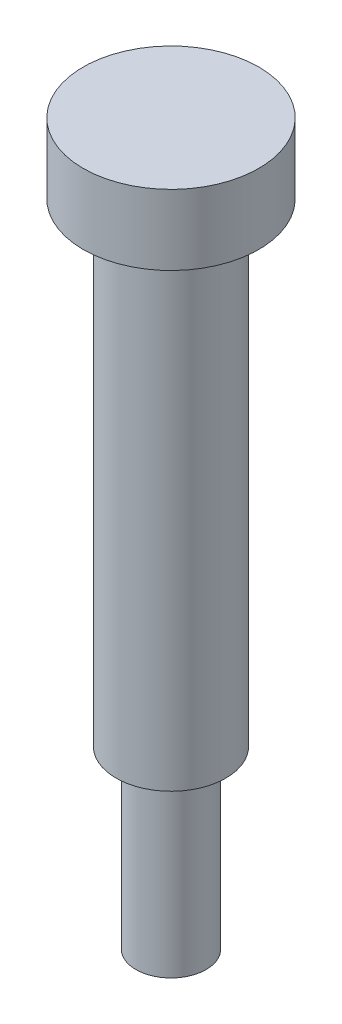
ISO-10303-21;
HEADER;
FILE_DESCRIPTION(('STEP AP214'),'2;1');
FILE_NAME('part.step','',(''),(''),'','','');
FILE_SCHEMA(('AUTOMOTIVE_DESIGN { 1 0 10303 214 1 1 1 1 }'));
ENDSEC;
DATA;
#1=APPLICATION_CONTEXT('core data for automotive mechanical design processes');
#2=APPLICATION_PROTOCOL_DEFINITION('international standard','automotive_design',2000,#1);
#3=PRODUCT_CONTEXT('',#1,'mechanical');
#4=PRODUCT('Part','Part','',(#3));
#5=PRODUCT_RELATED_PRODUCT_CATEGORY('part','',(#4));
#6=PRODUCT_DEFINITION_FORMATION('','',#4);
#7=PRODUCT_DEFINITION_CONTEXT('part definition',#1,'design');
#8=PRODUCT_DEFINITION('design','',#6,#7);
#9=PRODUCT_DEFINITION_SHAPE('','',#8);
#10=(LENGTH_UNIT() NAMED_UNIT(*) SI_UNIT(.MILLI.,.METRE.));
#11=(NAMED_UNIT(*) PLANE_ANGLE_UNIT() SI_UNIT($,.RADIAN.));
#12=(NAMED_UNIT(*) SI_UNIT($,.STERADIAN.) SOLID_ANGLE_UNIT());
#13=UNCERTAINTY_MEASURE_WITH_UNIT(LENGTH_MEASURE(1.E-05),#10,'distance_accuracy_value','');
#14=(GEOMETRIC_REPRESENTATION_CONTEXT(3) GLOBAL_UNCERTAINTY_ASSIGNED_CONTEXT((#13)) GLOBAL_UNIT_ASSIGNED_CONTEXT((#10,
#11,#12)) REPRESENTATION_CONTEXT('',''));
#15=CARTESIAN_POINT('',(0.,0.,0.));
#16=DIRECTION('',(0.,0.,1.));
#17=DIRECTION('',(1.,0.,0.));
#18=AXIS2_PLACEMENT_3D('',#15,#16,#17);
#19=CARTESIAN_POINT('',(0.,41.,0.));
#20=DIRECTION('',(0.,-1.,0.));
#21=DIRECTION('',(0.,0.,-1.));
#22=AXIS2_PLACEMENT_3D('',#19,#20,#21);
#23=PLANE('',#22);
#24=CARTESIAN_POINT('',(0.,41.,0.));
#25=DIRECTION('',(0.,-1.,0.));
#26=DIRECTION('',(0.,0.,-1.));
#27=AXIS2_PLACEMENT_3D('',#24,#25,#26);
#28=CIRCLE('',#27,5.);
#29=CARTESIAN_POINT('',(0.,41.,-5.));
#30=VERTEX_POINT('',#29);
#31=EDGE_CURVE('E10',#30,#30,#28,.T.);
#32=ORIENTED_EDGE('',*,*,#31,.F.);
#33=EDGE_LOOP('',(#32));
#34=FACE_BOUND('',#33,.T.);
#35=ADVANCED_FACE('F41',(#34),#23,.F.);
#36=CARTESIAN_POINT('',(0.,0.,0.));
#37=DIRECTION('',(0.,-1.,0.));
#38=DIRECTION('',(0.,0.,-1.));
#39=AXIS2_PLACEMENT_3D('',#36,#37,#38);
#40=CYLINDRICAL_SURFACE('',#39,5.);
#41=CARTESIAN_POINT('',(0.,37.,0.));
#42=DIRECTION('',(0.,-1.,0.));
#43=DIRECTION('',(0.,0.,-1.));
#44=AXIS2_PLACEMENT_3D('',#41,#42,#43);
#45=CIRCLE('',#44,5.);
#46=CARTESIAN_POINT('',(0.,37.,-5.));
#47=VERTEX_POINT('',#46);
#48=EDGE_CURVE('E50',#47,#47,#45,.T.);
#49=ORIENTED_EDGE('',*,*,#48,.F.);
#50=EDGE_LOOP('',(#49));
#51=FACE_BOUND('',#50,.T.);
#52=ORIENTED_EDGE('',*,*,#31,.T.);
#53=EDGE_LOOP('',(#52));
#54=FACE_BOUND('',#53,.T.);
#55=ADVANCED_FACE('F90',(#51,#54),#40,.T.);
#56=CARTESIAN_POINT('',(-3.125,37.,0.));
#57=DIRECTION('',(0.,1.,0.));
#58=DIRECTION('',(0.,0.,1.));
#59=AXIS2_PLACEMENT_3D('',#56,#57,#58);
#60=PLANE('',#59);
#61=CARTESIAN_POINT('',(0.,37.,0.));
#62=DIRECTION('',(0.,-1.,0.));
#63=DIRECTION('',(0.,0.,-1.));
#64=AXIS2_PLACEMENT_3D('',#61,#62,#63);
#65=CIRCLE('',#64,3.125);
#66=CARTESIAN_POINT('',(0.,37.,-3.125));
#67=VERTEX_POINT('',#66);
#68=EDGE_CURVE('E51',#67,#67,#65,.T.);
#69=ORIENTED_EDGE('',*,*,#68,.F.);
#70=EDGE_LOOP('',(#69));
#71=FACE_BOUND('',#70,.T.);
#72=ORIENTED_EDGE('',*,*,#48,.T.);
#73=EDGE_LOOP('',(#72));
#74=FACE_BOUND('',#73,.T.);
#75=ADVANCED_FACE('F83',(#71,#74),#60,.F.);
#76=CARTESIAN_POINT('',(0.,0.,0.));
#77=DIRECTION('',(0.,-1.,0.));
#78=DIRECTION('',(0.,0.,-1.));
#79=AXIS2_PLACEMENT_3D('',#76,#77,#78);
#80=CYLINDRICAL_SURFACE('',#79,3.125);
#81=CARTESIAN_POINT('',(0.,10.,0.));
#82=DIRECTION('',(0.,-1.,0.));
#83=DIRECTION('',(0.,0.,-1.));
#84=AXIS2_PLACEMENT_3D('',#81,#82,#83);
#85=CIRCLE('',#84,3.125);
#86=CARTESIAN_POINT('',(0.,10.,-3.125));
#87=VERTEX_POINT('',#86);
#88=EDGE_CURVE('E54',#87,#87,#85,.T.);
#89=ORIENTED_EDGE('',*,*,#88,.F.);
#90=EDGE_LOOP('',(#89));
#91=FACE_BOUND('',#90,.T.);
#92=ORIENTED_EDGE('',*,*,#68,.T.);
#93=EDGE_LOOP('',(#92));
#94=FACE_BOUND('',#93,.T.);
#95=ADVANCED_FACE('F79',(#91,#94),#80,.T.);
#96=CARTESIAN_POINT('',(-2.,10.,0.));
#97=DIRECTION('',(0.,1.,0.));
#98=DIRECTION('',(0.,0.,1.));
#99=AXIS2_PLACEMENT_3D('',#96,#97,#98);
#100=PLANE('',#99);
#101=CARTESIAN_POINT('',(0.,10.,0.));
#102=DIRECTION('',(0.,-1.,0.));
#103=DIRECTION('',(0.,0.,-1.));
#104=AXIS2_PLACEMENT_3D('',#101,#102,#103);
#105=CIRCLE('',#104,2.);
#106=CARTESIAN_POINT('',(0.,10.,-2.));
#107=VERTEX_POINT('',#106);
#108=EDGE_CURVE('E58',#107,#107,#105,.T.);
#109=ORIENTED_EDGE('',*,*,#108,.F.);
#110=EDGE_LOOP('',(#109));
#111=FACE_BOUND('',#110,.T.);
#112=ORIENTED_EDGE('',*,*,#88,.T.);
#113=EDGE_LOOP('',(#112));
#114=FACE_BOUND('',#113,.T.);
#115=ADVANCED_FACE('F75',(#111,#114),#100,.F.);
#116=CARTESIAN_POINT('',(0.,0.,0.));
#117=DIRECTION('',(0.,-1.,0.));
#118=DIRECTION('',(0.,0.,-1.));
#119=AXIS2_PLACEMENT_3D('',#116,#117,#118);
#120=CYLINDRICAL_SURFACE('',#119,2.);
#121=CARTESIAN_POINT('',(0.,0.,0.));
#122=DIRECTION('',(0.,-1.,0.));
#123=DIRECTION('',(0.,0.,-1.));
#124=AXIS2_PLACEMENT_3D('',#121,#122,#123);
#125=CIRCLE('',#124,2.);
#126=CARTESIAN_POINT('',(0.,0.,-2.));
#127=VERTEX_POINT('',#126);
#128=EDGE_CURVE('E64',#127,#127,#125,.T.);
#129=ORIENTED_EDGE('',*,*,#128,.F.);
#130=EDGE_LOOP('',(#129));
#131=FACE_BOUND('',#130,.T.);
#132=ORIENTED_EDGE('',*,*,#108,.T.);
#133=EDGE_LOOP('',(#132));
#134=FACE_BOUND('',#133,.T.);
#135=ADVANCED_FACE('F68',(#131,#134),#120,.T.);
#136=CARTESIAN_POINT('',(0.,0.,0.));
#137=DIRECTION('',(0.,1.,0.));
#138=DIRECTION('',(0.,0.,1.));
#139=AXIS2_PLACEMENT_3D('',#136,#137,#138);
#140=PLANE('',#139);
#141=ORIENTED_EDGE('',*,*,#128,.T.);
#142=EDGE_LOOP('',(#141));
#143=FACE_BOUND('',#142,.T.);
#144=ADVANCED_FACE('F67',(#143),#140,.F.);
#145=CLOSED_SHELL('',(#35,#55,#75,#95,#115,#135,#144));
#146=MANIFOLD_SOLID_BREP('B2',#145);
#147=ADVANCED_BREP_SHAPE_REPRESENTATION('',(#18,#146),#14);
#148=SHAPE_DEFINITION_REPRESENTATION(#9,#147);
ENDSEC;
END-ISO-10303-21;
